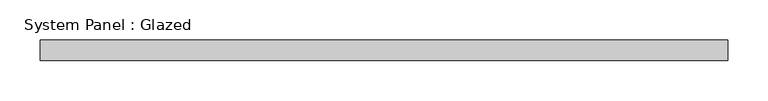
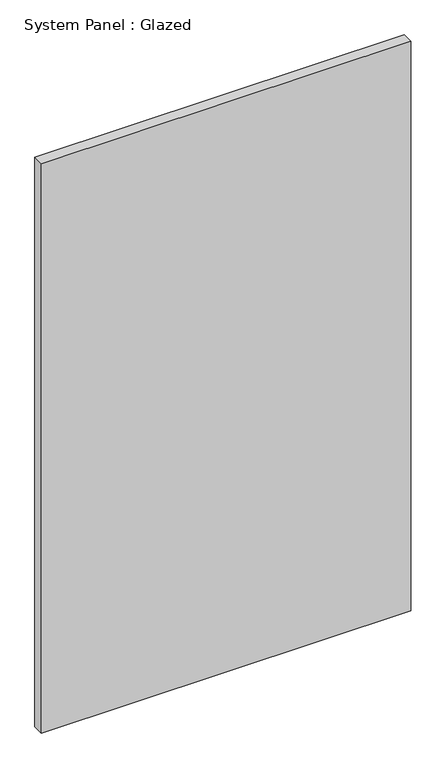
"""IFC4 building model written with IfcOpenShell, lengths in millimetres: plate geometry, System Panel : Glazed."""

from ifc_helpers import new_model, si_unit, origin, origin_with_axes, place, context, project, spatial, polyline, outline, extrude, source, transform, mapped, element, save


def system_panel_glazed_3a3afa19(model_context):
    return source(origin(), model_context, "Body", "SweptSolid", [
        extrude(outline(polyline([(425.45, 19.05), (-425.45, 19.05), (-425.45, 44.45), (425.45, 44.45), (425.45, 19.05)])), origin_with_axes(), (0.0, 0.0, 1.0), 1386.786396),
    ])


if __name__ == "__main__":
    model = new_model("IFC4")
    model_context = context("Model", 3, world=origin())
    ifc_project = project(units=[si_unit("LENGTHUNIT", "METRE", prefix="MILLI")], contexts=[model_context])
    site = spatial("IfcSite", under=ifc_project)
    building = spatial("IfcBuilding", under=site)
    placement = place(None, origin())
    system_panel_glazed_shape = system_panel_glazed_3a3afa19(model_context)
    element("IfcPlate", 1, ObjectType="System Panel : Glazed", at=placement, inside=building, context=model_context, shape_type="MappedRepresentation", body=[
        mapped(system_panel_glazed_shape, transform((0.0, 0.0, 0.0), x_axis=(1.0, 0.0, 0.0), y_axis=(0.0, 1.0, 0.0), z_axis=(0.0, 0.0, 1.0))),
    ])
    save(model, "model.ifc")

# Revit data of these elements
# Type "System Panel : Glazed"
#   Construction Type Id = "GSP4R"
#   Analytic Construction = "1/8 in Pilkington single glazing"
#   Visual Light Transmittance = 0.9
#   Solar Heat Gain Coefficient = 0.86
#   Heat Transfer Coefficient (U) = 1.18115 BTU/(h·ft²·°F)
#   Define Thermal Properties by = 1
# Element 1 (IfcPlate, "System Panel : Glazed")
#   Materials on its faces: "Glass"
# Materials
#   "Glass": class "Glass", colour RGB 0 128 192, transparency 0.75, Description = "Soda Lime Glass", Cost = 0
